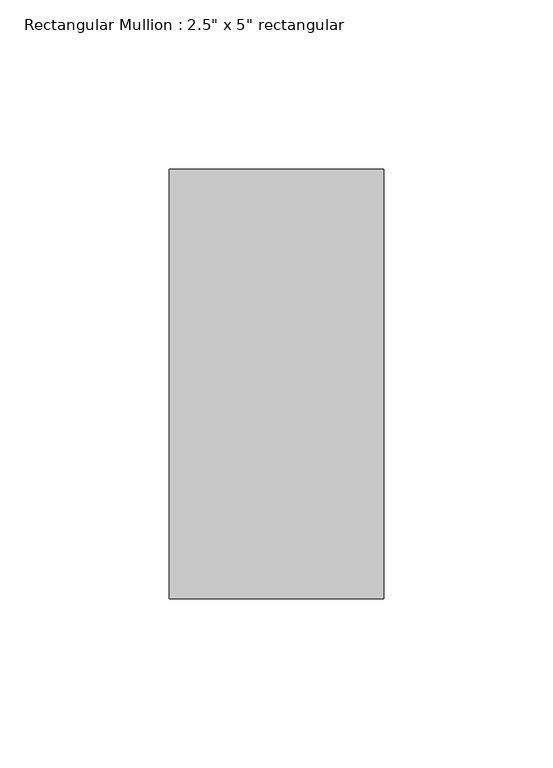
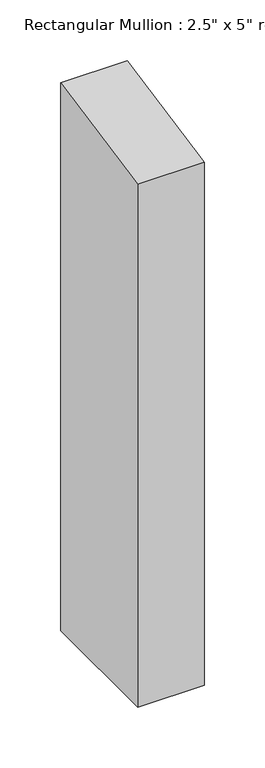
"""IFC4 building model written with IfcOpenShell, lengths in millimetres: member geometry."""

from ifc_helpers import new_model, si_unit, frame, origin, place, context, project, spatial, polyline, outline, extrude, source, transform, mapped, element, save


def member_55924089(model_context):
    return source(origin(), model_context, "Body", "SweptSolid", [
        extrude(outline(polyline([(-63.5, -12.6309353), (63.5, 12.6309353), (63.5, -539.4273751), (-63.5, -539.4273751), (-63.5, -12.6309353)])), frame((-63.5, 0.0, 0.0), z_axis=(1.0, 0.0, 0.0), x_axis=(0.0, 1.0, 0.0)), (0.0, 0.0, 1.0), 63.5),
    ])


if __name__ == "__main__":
    model = new_model("IFC4")
    model_context = context("Model", 3, world=origin())
    ifc_project = project(units=[si_unit("LENGTHUNIT", "METRE", prefix="MILLI")], contexts=[model_context])
    site = spatial("IfcSite", under=ifc_project)
    building = spatial("IfcBuilding", under=site)
    placement = place(None, origin())
    member_shape = member_55924089(model_context)
    element("IfcMember", 1, ObjectType="Rectangular Mullion : 2.5\" x 5\" rectangular", at=placement, inside=building, context=model_context, shape_type="MappedRepresentation", body=[
        mapped(member_shape, transform((0.0, 0.0, 0.0), x_axis=(1.0, 0.0, 0.0), y_axis=(0.0, 1.0, 0.0), z_axis=(0.0, 0.0, 1.0))),
    ])
    save(model, "model.ifc")

# Revit data of these elements
# Type "Rectangular Mullion : 2.5\" x 5\" rectangular"
#   built-in parameter 1007304 = 0.416667 (stored number, unit not read)
#   built-in parameter 1007301 = 0.104167 (stored number, unit not read)
#   built-in parameter 1007300 = 0.104167 (stored number, unit not read)
# Element 1 (IfcMember, "Rectangular Mullion : 2.5\" x 5\" rectangular")
#   Materials on its faces: "Iron, Ductile"
# Materials
#   "Iron, Ductile": class "Metal", colour RGB 0 0 0, transparency 0, Description = "Ductile cast iron", Cost = 0
